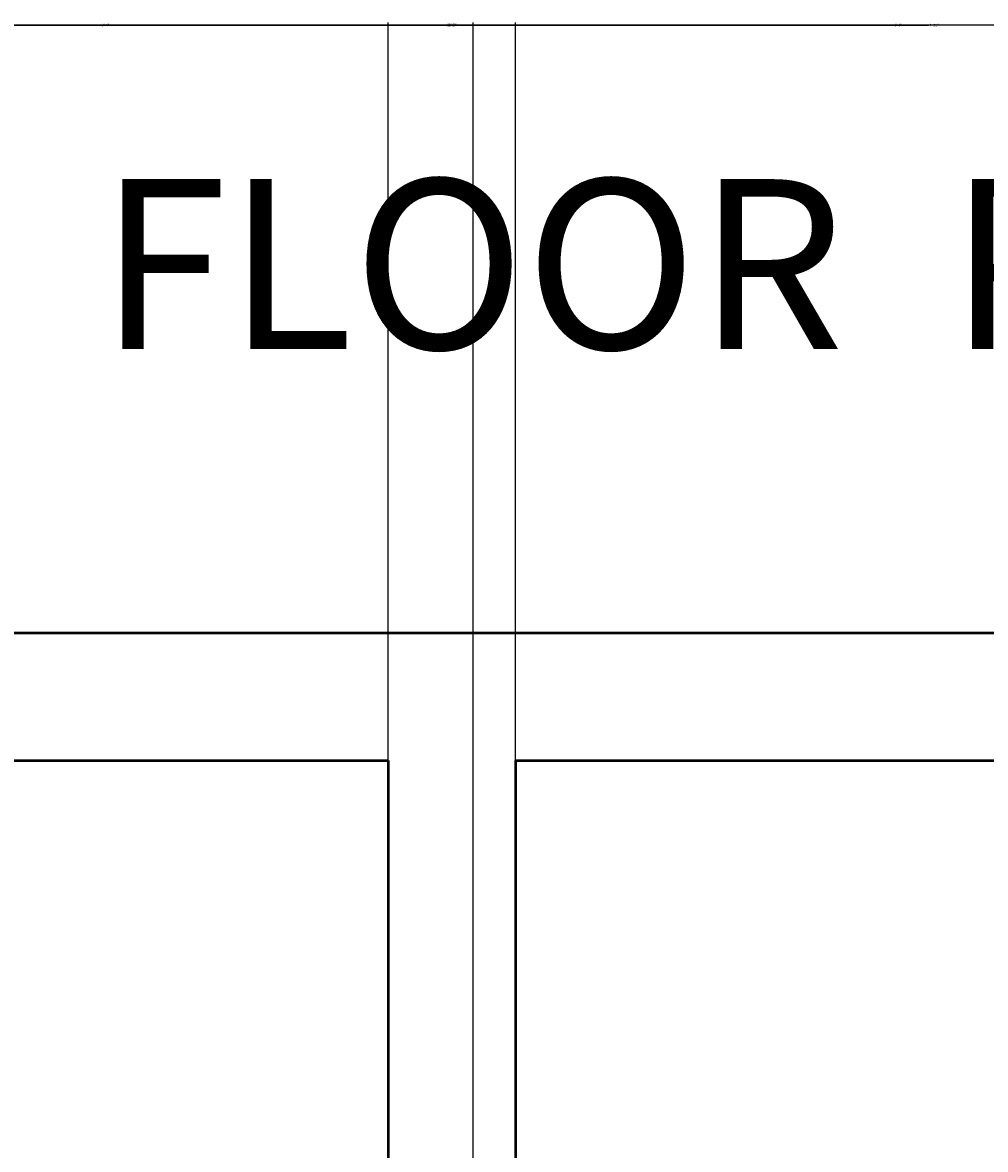
# Model space of a CAD drawing. Units: inches. Extents: x 37 to 824, y -700 to 234.
# Tile 69 of 77: x 264 to 332, y 155 to 234. Entities that reach past the tile are written whole.
import ezdxf

# ---------------------------------------------------------------- set-up
doc = ezdxf.new("R2010")
doc.units = ezdxf.units.IN
doc.header["$MEASUREMENT"] = 0
for name, color, linetype, lineweight in [('A-ANNO-DIMS', 2, 'Continuous', 18), ('A-ANNO-TEXT', 7, 'Continuous', 18), ('A-WALL', 2, 'Continuous', 50)]:
    doc.layers.add(name, color=color, linetype=linetype, lineweight=lineweight)
doc.styles.get("Standard").update_dxf_attribs({"font": 'arial.ttf'})
doc.dimstyles.get("Standard").update_dxf_attribs({"dimtxt": 0.18, "dimasz": 0.18, "dimexe": 0.18, "dimexo": 0.0625, "dimgap": 0.09, "dimtad": 0, "dimtih": 1, "dimtoh": 1, "dimdec": 1, "dimzin": 0, "dimdsep": 46, "dimlunit": 4, "dimtxsty": 'Standard', "dimcen": 0.09, "dimadec": 0, "dimazin": 0, "dimtfac": 1, "dimtdec": 1, "dimtofl": 0, "dimtmove": 0, "dimatfit": 3, "dimfxl": 1, "dimtolj": 1, "dimtzin": 0, "dimarcsym": 0})

# ---------------------------------------------------------------- blocks, each defined once
blk = doc.blocks.new('*D46')
at = {"layer": 'A-ANNO-DIMS', "color": 0, "lineweight": -2, "ltscale": 0.5, "transparency": 16777216}
for p, q in [((250.077, 191.153), (250.077, 234.17)), ((250.257, 233.99), (294.249, 233.99)), ((338.897, 233.99), (294.906, 233.99)), ((339.077, 191.153), (339.077, 234.17))]:
    blk.add_line(p, q, dxfattribs=at)
at = {"layer": 'A-ANNO-DIMS', "color": 0, "ltscale": 0.5, "transparency": 16777216}
for points in [[(250.257, 234.02), (250.257, 233.96), (250.077, 233.99)], [(338.897, 234.02), (338.897, 233.96), (339.077, 233.99)]]:
    blk.add_solid(points, dxfattribs=at)
at = {"layer": 'Defpoints', "color": 0, "ltscale": 0.5, "transparency": 16777216}
for p in [(339.077, 233.99), (250.077, 191.09), (339.077, 191.09)]:
    blk.add_point(p, dxfattribs=at)
at = {"layer": 'A-ANNO-DIMS', "color": 0, "ltscale": 0.5, "transparency": 16777216, "insert": (294.577, 233.99), "char_height": 0.18, "attachment_point": 5}
blk.add_mtext('\\A1;7\'-5"', dxfattribs=at)
blk = doc.blocks.new('*D63')
at = {"layer": 'A-ANNO-DIMS', "color": 0, "lineweight": -2, "ltscale": 0.5, "transparency": 16777216}
for p, q in [((161.077, 191.153), (161.077, 234.17)), ((161.257, 233.99), (294.176, 233.99)), ((427.897, 233.99), (294.978, 233.99)), ((428.077, 191.153), (428.077, 234.17))]:
    blk.add_line(p, q, dxfattribs=at)
at = {"layer": 'A-ANNO-DIMS', "color": 0, "ltscale": 0.5, "transparency": 16777216}
for points in [[(161.257, 234.02), (161.257, 233.96), (161.077, 233.99)], [(427.897, 234.02), (427.897, 233.96), (428.077, 233.99)]]:
    blk.add_solid(points, dxfattribs=at)
at = {"layer": 'Defpoints', "color": 0, "ltscale": 0.5, "transparency": 16777216}
for p in [(428.077, 233.99), (161.077, 191.09), (428.077, 191.09)]:
    blk.add_point(p, dxfattribs=at)
at = {"layer": 'A-ANNO-DIMS', "color": 0, "ltscale": 0.5, "transparency": 16777216, "insert": (294.577, 233.99), "char_height": 0.18, "attachment_point": 5}
blk.add_mtext('\\A1;22\'-3"', dxfattribs=at)
blk = doc.blocks.new('*D73')
at = {"layer": 'A-ANNO-DIMS', "color": 0, "lineweight": -2, "ltscale": 0.5, "transparency": 16777216}
for p, q in [((250.19, 84.153), (250.19, 234.17)), ((250.37, 233.99), (269.804, 233.99)), ((289.897, 233.99), (270.463, 233.99)), ((290.077, 81.153), (290.077, 234.17))]:
    blk.add_line(p, q, dxfattribs=at)
at = {"layer": 'A-ANNO-DIMS', "color": 0, "ltscale": 0.5, "transparency": 16777216}
for points in [[(250.37, 234.02), (250.37, 233.96), (250.19, 233.99)], [(289.897, 234.02), (289.897, 233.96), (290.077, 233.99)]]:
    blk.add_solid(points, dxfattribs=at)
at = {"layer": 'Defpoints', "color": 0, "ltscale": 0.5, "transparency": 16777216}
for p in [(290.077, 233.99), (250.19, 84.09), (290.077, 81.09)]:
    blk.add_point(p, dxfattribs=at)
at = {"layer": 'A-ANNO-DIMS', "color": 0, "ltscale": 0.5, "transparency": 16777216, "insert": (270.133, 233.99), "char_height": 0.18, "attachment_point": 5}
blk.add_mtext('\\A1;3\'-4"', dxfattribs=at)
blk = doc.blocks.new('*D78')
at = {"layer": 'A-ANNO-DIMS', "color": 0, "lineweight": -2, "ltscale": 0.5, "transparency": 16777216}
for p, q in [((290.077, 15.153), (290.077, 234.17)), ((290.257, 233.99), (325.747, 233.99)), ((361.897, 233.99), (326.407, 233.99)), ((362.077, 15.153), (362.077, 234.17))]:
    blk.add_line(p, q, dxfattribs=at)
at = {"layer": 'A-ANNO-DIMS', "color": 0, "ltscale": 0.5, "transparency": 16777216}
for points in [[(290.257, 234.02), (290.257, 233.96), (290.077, 233.99)], [(361.897, 234.02), (361.897, 233.96), (362.077, 233.99)]]:
    blk.add_solid(points, dxfattribs=at)
at = {"layer": 'Defpoints', "color": 0, "ltscale": 0.5, "transparency": 16777216}
for p in [(362.077, 233.99), (290.077, 15.09), (362.077, 15.09)]:
    blk.add_point(p, dxfattribs=at)
at = {"layer": 'A-ANNO-DIMS', "color": 0, "ltscale": 0.5, "transparency": 16777216, "insert": (326.077, 233.99), "char_height": 0.18, "attachment_point": 5}
blk.add_mtext('\\A1;6\'-0"', dxfattribs=at)
blk = doc.blocks.new('*D82')
at = {"layer": 'A-ANNO-DIMS', "color": 0, "lineweight": -2, "ltscale": 0.5, "transparency": 16777216}
for p, q in [((299.077, -206.847), (299.077, 234.17)), ((299.257, 233.99), (328.202, 233.99)), ((357.952, 233.99), (329.008, 233.99)), ((358.132, -206.847), (358.132, 234.17))]:
    blk.add_line(p, q, dxfattribs=at)
at = {"layer": 'A-ANNO-DIMS', "color": 0, "ltscale": 0.5, "transparency": 16777216}
for points in [[(299.257, 234.02), (299.257, 233.96), (299.077, 233.99)], [(357.952, 234.02), (357.952, 233.96), (358.132, 233.99)]]:
    blk.add_solid(points, dxfattribs=at)
at = {"layer": 'Defpoints', "color": 0, "ltscale": 0.5, "transparency": 16777216}
for p in [(358.132, 233.99), (299.077, -206.91), (358.132, -206.91)]:
    blk.add_point(p, dxfattribs=at)
at = {"layer": 'A-ANNO-DIMS', "color": 0, "ltscale": 0.5, "transparency": 16777216, "insert": (328.605, 233.99), "char_height": 0.18, "attachment_point": 5}
blk.add_mtext('\\A1;4\'-11"', dxfattribs=at)
blk = doc.blocks.new('*D87')
at = {"layer": 'A-ANNO-DIMS', "color": 0, "lineweight": -2, "ltscale": 0.5, "transparency": 16777216}
for p, q in [((216.077, -356.847), (216.077, 234.17)), ((216.257, 233.99), (255.747, 233.99)), ((295.897, 233.99), (256.407, 233.99)), ((296.077, -356.847), (296.077, 234.17))]:
    blk.add_line(p, q, dxfattribs=at)
at = {"layer": 'A-ANNO-DIMS', "color": 0, "ltscale": 0.5, "transparency": 16777216}
for points in [[(216.257, 234.02), (216.257, 233.96), (216.077, 233.99)], [(295.897, 234.02), (295.897, 233.96), (296.077, 233.99)]]:
    blk.add_solid(points, dxfattribs=at)
at = {"layer": 'Defpoints', "color": 0, "ltscale": 0.5, "transparency": 16777216}
for p in [(296.077, 233.99), (216.077, -356.91), (296.077, -356.91)]:
    blk.add_point(p, dxfattribs=at)
at = {"layer": 'A-ANNO-DIMS', "color": 0, "ltscale": 0.5, "transparency": 16777216, "insert": (256.077, 233.99), "char_height": 0.18, "attachment_point": 5}
blk.add_mtext('\\A1;6\'-8"', dxfattribs=at)

msp = doc.modelspace()

# ---------------------------------------------------------------- linework, layer by layer
at = {"layer": 'A-WALL'}
for p, q in [((161.077, 191.09), (299.077, 191.09)), ((299.077, 191.09), (428.077, 191.09)), ((170.077, 182.09), (290.077, 182.09)), ((290.077, 182.09), (290.077, 75.09)), ((299.077, 182.09), (299.077, 75.09)), ((299.077, 182.09), (419.077, 182.09))]:
    msp.add_line(p, q, dxfattribs=at)

# ---------------------------------------------------------------- texts
at = {"layer": 'A-ANNO-TEXT'}
msp.add_text('GROUND  FLOOR  PLAN', height=12, dxfattribs=at).set_placement((193.612, 211.117))

# ---------------------------------------------------------------- dimensions: what is measured, and where the dimension line sits
at = {"layer": 'A-ANNO-DIMS', "ltscale": 0.5}
for base, p1, p2, picture, middle in [((428.077, 233.99), (161.077, 191.09), (428.077, 191.09), '*D63', (294.577, 233.99)), ((296.077, 233.99), (216.077, -356.91), (296.077, -356.91), '*D87', (256.077, 233.99)), ((339.077, 233.99), (250.077, 191.09), (339.077, 191.09), '*D46', (294.577, 233.99)), ((290.077, 233.99), (250.19, 84.09), (290.077, 81.09), '*D73', (270.133, 233.99)), ((362.077, 233.99), (290.077, 15.09), (362.077, 15.09), '*D78', (326.077, 233.99)), ((358.132, 233.99), (299.077, -206.91), (358.132, -206.91), '*D82', (328.605, 233.99))]:
    dim = msp.add_linear_dim(base=base, p1=p1, p2=p2, dimstyle='Standard', override={"dimdec": 1, "dimlfac": 1, "dimrnd": 0, "dimzin": 1, "dimdsep": 46, "dimlunit": 4, "dimfrac": 2}, dxfattribs=at)
    dim.commit()
    dim.dimension.update_dxf_attribs({"geometry": picture, "text_midpoint": middle})

doc.saveas('drawing.dxf')
